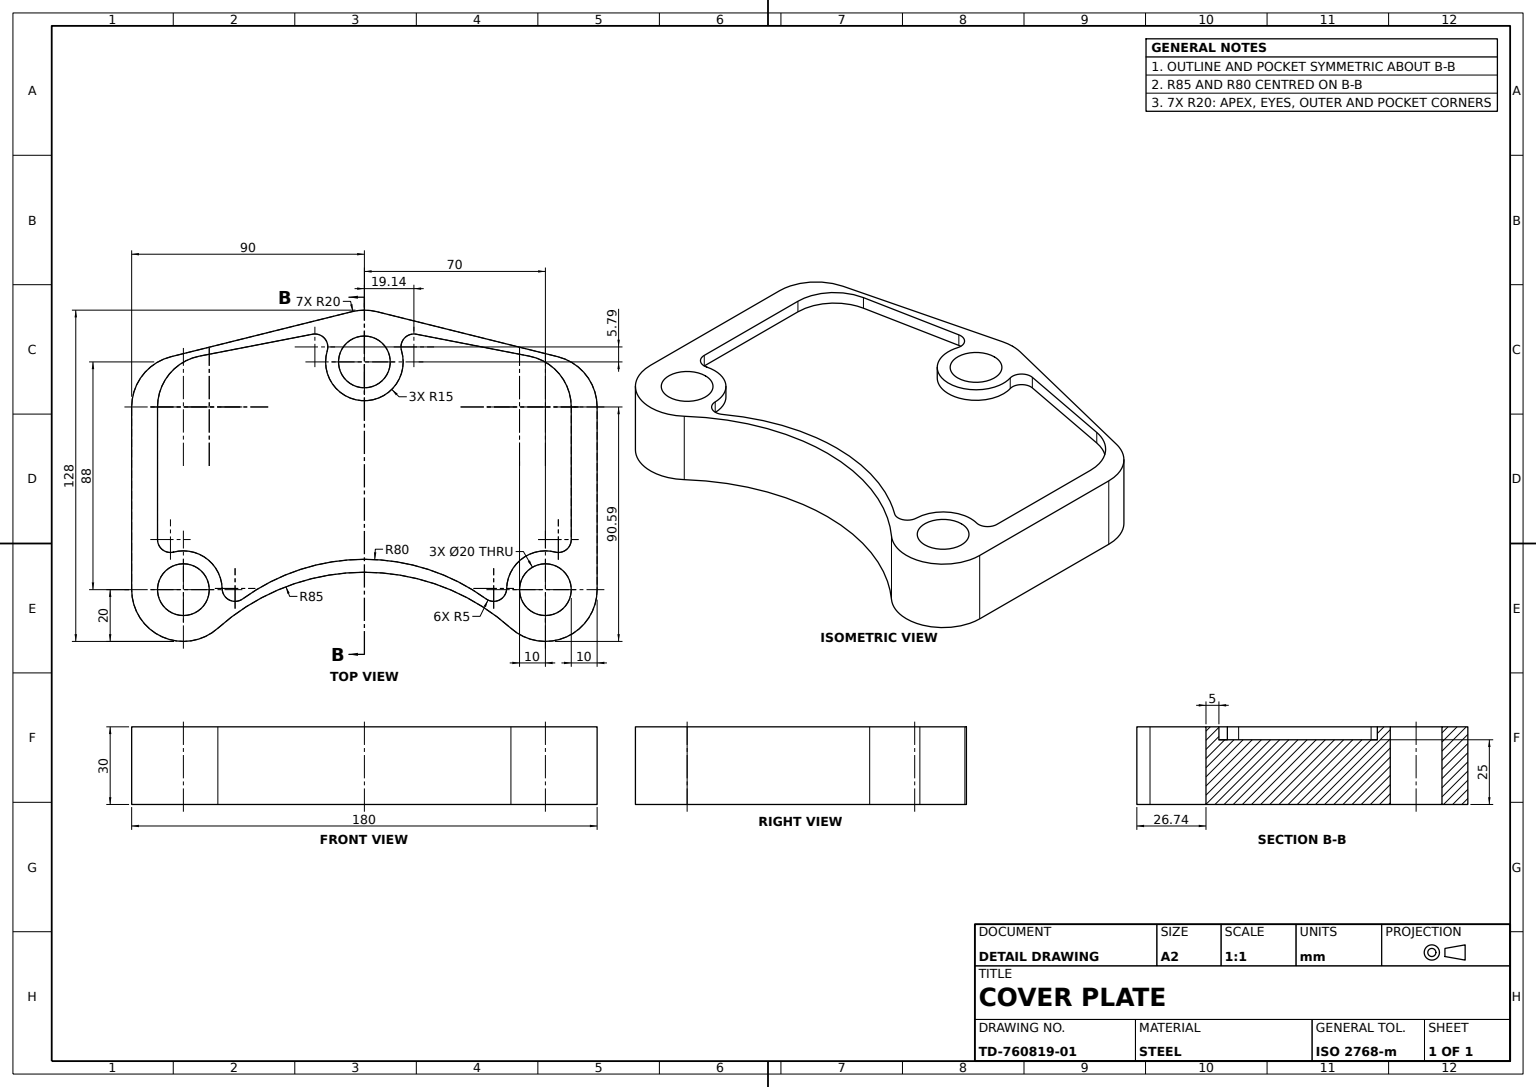
SolidWorks part; units mm, degrees
material "Plain Carbon Steel"
ref_plane "Front Plane" through (0, 0, 0) normal (0, 0, 1) x (1, 0, 0)
ref_plane "Top Plane" through (0, 0, 0) normal (0, 1, 0) x (1, 0, 0)
ref_plane "Right Plane" through (0, 0, 0) normal (1, 0, 0) x (0, 0, -1)
sketch "Plate Outline Sketch" plane through (0, 0, 0) normal (0, 1, 0) x (1, 0, 0)
  line L0 (0, 0) -> (0, -126.9357) construction
  line L1 (-90, -88) -> (-90, -17.4088)
  line L2 (-74.8269, 2) -> (-4.8269, 19.4088)
  line L3 (-80, -68.6351) -> (-80, -17.4088)
  line L4 (-63.8045, 2.226) -> (-20.0957, 10.6952)
  line L5 (63.8045, 2.226) -> (20.0957, 10.6952)
  line L6 (74.8269, 2) -> (4.8269, 19.4088)
  line L7 (90, -88) -> (90, -17.4088)
  line L8 (80, -68.6351) -> (80, -17.4088)
  arc A0 (4.8269, 19.4088) -> (-4.8269, 19.4088) centre (0, 0) ccw
  circle A1 centre (0, 0) radius 10
  arc A2 (-90, -88) -> (-56.6667, -102.9071) centre (-70, -88) ccw
  circle A3 centre (-70, -88) radius 10
  arc A4 (-55.0042, -87.6458) -> (-73.75, -73.4763) centre (-70, -88) ccw
  arc A5 (-90, -17.4088) -> (-74.8269, 2) centre (-70, -17.4088) cw
  arc A6 (-14.3585, 4.3399) -> (14.3585, 4.3399) centre (0, 0) ccw
  arc A7 (-73.75, -73.4763) -> (-80, -68.6351) centre (-75, -68.6351) cw
  arc A8 (-80, -17.4088) -> (-63.8045, 2.226) centre (-60, -17.4088) cw
  arc A9 (-20.0957, 10.6952) -> (-14.3585, 4.3399) centre (-19.1446, 5.7865) cw
  arc A10 (20.0957, 10.6952) -> (14.3585, 4.3399) centre (19.1446, 5.7865) ccw
  arc A11 (90, -17.4088) -> (74.8269, 2) centre (70, -17.4088) ccw
  arc A12 (80, -17.4088) -> (63.8045, 2.226) centre (60, -17.4088) ccw
  arc A13 (73.75, -73.4763) -> (80, -68.6351) centre (75, -68.6351) ccw
  circle A14 centre (70, -88) radius 10
  arc A15 (55.0042, -87.6458) -> (73.75, -73.4763) centre (70, -88) cw
  arc A16 (90, -88) -> (56.6667, -102.9071) centre (70, -88) cw
  arc A17 (-55.0042, -87.6458) -> (-47.0641, -91.571) centre (-50.0056, -87.5278) ccw
  arc A18 (-47.0641, -91.571) -> (47.0641, -91.571) centre (0, -156.2624) cw
  arc A19 (47.0641, -91.571) -> (55.0042, -87.6458) centre (50.0056, -87.5278) ccw
  arc A20 (-56.6667, -102.9071) -> (56.6667, -102.9071) centre (0, -166.2624) cw
  point P6 (-80, -43.0219)
  point P47 (0, -76.2624)
  dimension "D1" = 20
  dimension "D2" = 20
  dimension "D3" = 40
  dimension "D4" = 30
  dimension "D5" = 20
  dimension "D8" = 20
  dimension "D9" = 30
  dimension "D10" = 20
  dimension "D11" = 5
  dimension "D12" = 5
  dimension "D14" = 5
  dimension "D15" = 5
  dimension "D16" = 10
  dimension "D17" = 10
  dimension "D18" = 3
  dimension "D19" = 85
  dimension "D20" = 80
  dimension "D6" = 88
  dimension "D7" = 70
  dimension "D13" = 90
extrude "Base Plate 30mm" add sketch "Plate Outline Sketch" along normal blind 30
sketch "Top Pocket Sketch" plane through (0, 0, 0) normal (0, -1, 0) x (1, 0, 0)
  line L0 (-20.0957, -10.6952) -> (-63.8045, -2.226) construction
  line L1 (63.8045, -2.226) -> (20.0957, -10.6952) construction
  line L2 (80, 68.6351) -> (80, 17.4088) construction
  line L3 (-80, 17.4088) -> (-80, 68.6351) construction
  line L4 (-20.0957, -10.6952) -> (-63.8045, -2.226)
  line L5 (63.8045, -2.226) -> (20.0957, -10.6952)
  line L6 (80, 68.6351) -> (80, 17.4088)
  line L7 (-80, 17.4088) -> (-80, 68.6351)
  arc A0 (-80, 17.4088) -> (-63.8045, -2.226) centre (-60, 17.4088) ccw construction
  arc A1 (-20.0957, -10.6952) -> (-14.3585, -4.3399) centre (-19.1446, -5.7865) ccw construction
  arc A2 (14.3585, -4.3399) -> (-14.3585, -4.3399) centre (0, 0) ccw construction
  arc A3 (14.3585, -4.3399) -> (20.0957, -10.6952) centre (19.1446, -5.7865) ccw construction
  arc A4 (63.8045, -2.226) -> (80, 17.4088) centre (60, 17.4088) ccw construction
  arc A5 (80, 68.6351) -> (73.75, 73.4763) centre (75, 68.6351) ccw construction
  arc A6 (55.0042, 87.6458) -> (73.75, 73.4763) centre (70, 88) ccw construction
  arc A7 (55.0042, 87.6458) -> (47.0641, 91.571) centre (50.0056, 87.5278) ccw construction
  arc A8 (-73.75, 73.4763) -> (-80, 68.6351) centre (-75, 68.6351) ccw construction
  arc A9 (-47.0641, 91.571) -> (47.0641, 91.571) centre (0, 156.2624) ccw construction
  arc A10 (-47.0641, 91.571) -> (-55.0042, 87.6458) centre (-50.0056, 87.5278) ccw construction
  arc A11 (-73.75, 73.4763) -> (-55.0042, 87.6458) centre (-70, 88) ccw construction
  arc A12 (-80, 17.4088) -> (-63.8045, -2.226) centre (-60, 17.4088) ccw
  arc A13 (-20.0957, -10.6952) -> (-14.3585, -4.3399) centre (-19.1446, -5.7865) ccw
  arc A14 (14.3585, -4.3399) -> (-14.3585, -4.3399) centre (0, 0) ccw
  arc A15 (14.3585, -4.3399) -> (20.0957, -10.6952) centre (19.1446, -5.7865) ccw
  arc A16 (63.8045, -2.226) -> (80, 17.4088) centre (60, 17.4088) ccw
  arc A17 (80, 68.6351) -> (73.75, 73.4763) centre (75, 68.6351) ccw
  arc A18 (55.0042, 87.6458) -> (73.75, 73.4763) centre (70, 88) ccw
  arc A19 (55.0042, 87.6458) -> (47.0641, 91.571) centre (50.0056, 87.5278) ccw
  arc A20 (-73.75, 73.4763) -> (-80, 68.6351) centre (-75, 68.6351) ccw
  arc A21 (-47.0641, 91.571) -> (47.0641, 91.571) centre (0, 156.2624) ccw
  arc A22 (-47.0641, 91.571) -> (-55.0042, 87.6458) centre (-50.0056, 87.5278) ccw
  arc A23 (-73.75, 73.4763) -> (-55.0042, 87.6458) centre (-70, 88) ccw
extrude "Top Pocket Cut" add sketch "Top Pocket Sketch" against normal blind 25
